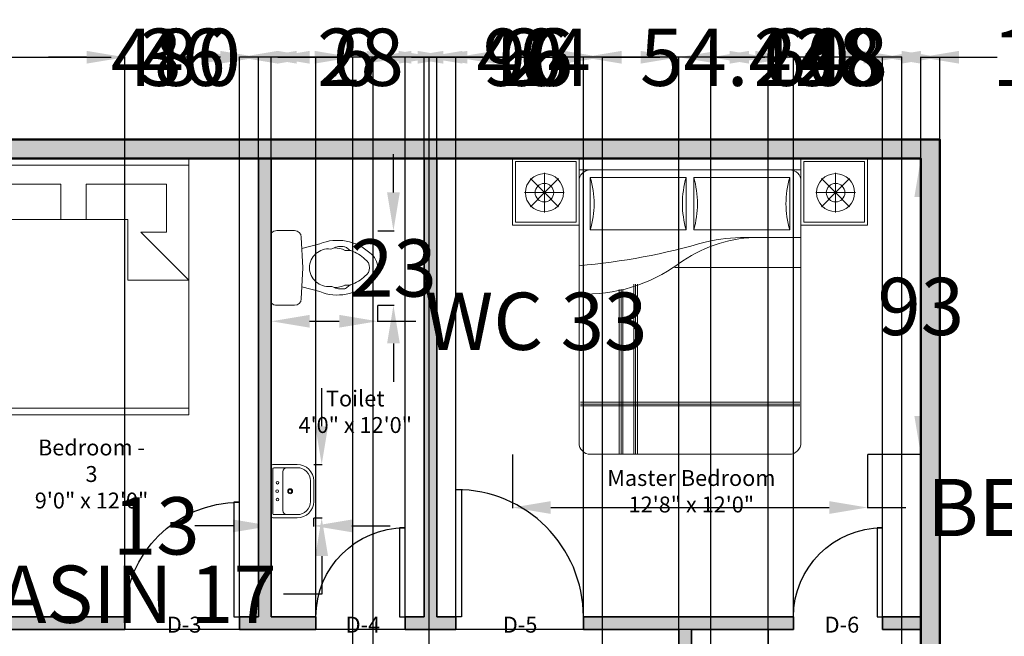
# Model space of a CAD drawing. Units: inches. Extents: x -478 to 256, y -93 to 343.
# Tile 4 of 5: x -211 to 98, y 149 to 343. Entities that reach past the tile are written whole.
import ezdxf

# ---------------------------------------------------------------- set-up
doc = ezdxf.new("R2010")
doc.units = ezdxf.units.IN
for name, color, linetype, lineweight in [('A-ANNO-DIMS', 2, 'Continuous', 18), ('A-ANNO-TEXT', 7, 'Continuous', 18), ('A-AREA-IDEN', 7, 'Continuous', 18), ('A-DOOR', 3, 'Continuous', 25), ('A-FLOR-CASE', 6, 'Continuous', 25), ('A-FLOR-FIXT', 9, 'Continuous', 18), ('A-WALL-PATT', 8, 'Continuous', 13), ('Furniture', 2, 'Continuous', 18), ('Inner Wall', 5, 'Continuous', 35), ('Outer Wall', 1, 'Continuous', 50)]:
    doc.layers.add(name, color=color, linetype=linetype, lineweight=lineweight)
doc.styles.get("Standard").update_dxf_attribs({"font": 'arial.ttf'})
doc.dimstyles.get("Standard").update_dxf_attribs({"dimtxt": 18, "dimasz": 12, "dimexe": 0.18, "dimexo": 0.0625, "dimgap": 0.09, "dimtad": 0, "dimtih": 1, "dimtoh": 1, "dimdec": 0, "dimzin": 0, "dimdsep": 46, "dimlunit": 3, "dimtxsty": 'Standard', "dimcen": 0.09, "dimadec": 0, "dimazin": 0, "dimtfac": 1, "dimtdec": 0, "dimtofl": 0, "dimtmove": 0, "dimatfit": 3, "dimfxl": 1, "dimtolj": 1, "dimtzin": 0, "dimarcsym": 0})

# ---------------------------------------------------------------- blocks, each defined once
blk = doc.blocks.new('*U2')
for p, q in [((0, 0), (0, -4)), ((36, 0), (36, -4))]:
    blk.add_line(p, q)
blk.add_lwpolyline([(0, 0), (0, 36), (1.75, 36), (1.75, 0)], close=True)
blk.add_arc((0, 0), 36, 0, 90)
blk = doc.blocks.new('*U3')
for p, q in [((0, 0), (0, -4)), ((40, 0), (40, -4))]:
    blk.add_line(p, q)
blk.add_lwpolyline([(0, 0), (0, 40), (1.75, 40), (1.75, 0)], close=True)
blk.add_arc((0, 0), 40, 0, 90)
blk = doc.blocks.new('*U4')
for p, q in [((0, 0), (0, -4)), ((28, 0), (28, -4))]:
    blk.add_line(p, q)
blk.add_lwpolyline([(0, 0), (0, 28), (1.75, 28), (1.75, 0)], close=True)
blk.add_arc((0, 0), 28, 0, 90)
blk = doc.blocks.new('A$C1308471B')
at = {"ltscale": 20}
for p, q in [((0, 0.4607), (0, 0.0186)), ((0.0354, 0.4793), (0.1495, 0.4793)), ((0.2013, 0.2397), (0.1923, 0.4384)), ((0.1957, 0.3639), (0.3109, 0.3953)), ((0.5021, 0.3528), (0.4724, 0.3528)), ((0.4982, 0.3575), (0.4822, 0.3709)), ((0.2013, 0.2397), (0.1923, 0.0409)), ((0.5021, 0.1304), (0.4724, 0.1304)), ((0.1959, 0.1193), (0.3109, 0.0879)), ((0.4982, 0.1257), (0.4822, 0.1123)), ((0.0354, 0), (0.1495, 0))]:
    blk.add_line(p, q, dxfattribs=at)
for centre, radius, start, end in [((0.006, 0.4607), 0.006, 136.52689, 180), ((0.0354, 0.4328), 0.0465, 90, 136.52689), ((0.1495, 0.4365), 0.0429, 2.57554, 90), ((0.4248, 0.1104), 0.3068, 47.41345, 111.79241), ((0.3654, 0.2416), 0.1206, 83.35226, 180), ((0.3823, 0.3868), 0.0255, 263.35226, 298.57415), ((0.4494, 0.2636), 0.1148, 79.39683, 118.57415), ((0.405, 0.2159), 0.153, 63.50202, 90.45216), ((0.4658, 0.3513), 0.0255, 50, 79.39683), ((0.5146, 0.377), 0.0255, 230, 251.38812), ((0.5021, 0.3273), 0.0255, 70.3751, 90), ((0.4248, 0.1104), 0.2558, 46.61198, 70.3751), ((0.5654, 0.2416), 0.116, 0, 54.71147), ((0.5654, 0.2416), 0.065, 0, 57.29738), ((0.3654, 0.2416), 0.1206, 180, 276.64774), ((0.5654, 0.2416), 0.065, 302.70262, 0), ((0.5654, 0.2416), 0.116, 305.28853, 0), ((0.4248, 0.3728), 0.3068, 248.20759, 312.58655), ((0.405, 0.2673), 0.153, 269.54784, 296.49798), ((0.5146, 0.1062), 0.0255, 108.61188, 130), ((0.5021, 0.1559), 0.0255, 270, 289.6249), ((0.4248, 0.3728), 0.2558, 289.6249, 313.38802), ((0.3823, 0.0964), 0.0255, 61.42585, 96.64774), ((0.4494, 0.2196), 0.1148, 241.42585, 280.60317), ((0.4658, 0.1319), 0.0255, 280.60317, 310), ((0.006, 0.0186), 0.006, 180, 223.47311), ((0.0354, 0.0465), 0.0465, 223.47311, 270), ((0.1495, 0.0429), 0.0429, 270, 357.42446)]:
    blk.add_arc(centre, radius, start, end, dxfattribs=at)
blk = doc.blocks.new('A$C57EA129C')
for p, q in [((0, 0.443), (0, 0.178)), ((0.016, 0.459), (0.563, 0.459)), ((0.036, 0.432), (0.036, 0.29)), ((0.045, 0.441), (0.535, 0.441)), ((0.544, 0.432), (0.544, 0.29)), ((0.579, 0.443), (0.579, 0.178)), ((0.08, 0.334), (0.499, 0.334)), ((0.036, 0.29), (0.036, 0.178)), ((0.544, 0.29), (0.544, 0.178)), ((0.178, 0.036), (0.401, 0.036)), ((0.178, 0), (0.401, 0))]:
    blk.add_line(p, q)
for centre, radius in [((0.198, 0.392), 0.0143), ((0.29, 0.396), 0.0156), ((0.381, 0.392), 0.0143), ((0.29, 0.255), 0.0267), ((0.29, 0.255), 0.0178)]:
    blk.add_circle(centre, radius)
for centre, radius, start, end in [((0.016, 0.443), 0.016, 90, 180), ((0.045, 0.432), 0.00891, 90, 180), ((0.535, 0.432), 0.00891, 0, 90), ((0.563, 0.443), 0.016, 0, 90), ((0.08, 0.29), 0.0445, 90, 180), ((0.499, 0.29), 0.0445, 0, 90), ((0.178, 0.178), 0.178, 180, 270), ((0.178, 0.178), 0.143, 180, 270), ((0.401, 0.178), 0.178, 270, 0), ((0.401, 0.178), 0.143, 270, 0)]:
    blk.add_arc(centre, radius, start, end)
blk = doc.blocks.new('KING-00')
for p, q in [((-0.8967, -0.947), (-0.8967, 0.8818)), ((0.6019, 0.8818), (0.6019, -0.4644)), ((1.0337, -0.947), (1.0337, 0.8818)), ((0.6019, 0.704), (0.8813, 0.704)), ((0.8813, 0.069), (0.8813, 0.704)), ((0.6019, 0.069), (0.8813, 0.069)), ((0.8813, -0.1342), (0.6019, -0.1342)), ((0.8813, -0.7692), (0.8813, -0.1342)), ((0.1193, -0.4644), (0.1193, -0.947)), ((0.6019, -0.4644), (0.1193, -0.4644)), ((0.1193, -0.947), (0.5003, -0.566)), ((0.5003, -0.7692), (0.5003, -0.566)), ((0.5003, -0.7692), (0.8813, -0.7692))]:
    blk.add_line(p, q)
blk.add_lwpolyline([(-0.9475, -0.947), (-0.9475, 0.8818), (1.0845, 0.8818), (1.0845, -0.947)], close=True)
blk = doc.blocks.new('A$C068671E6')
for p, q in [((0, 1.5502), (0, 2.0002)), ((0, 2.0002), (0.45, 2.0002)), ((0.45, 2.0002), (0.45, 1.5502)), ((1.9506, 2.0002), (1.9506, 1.5502)), ((2.4006, 2.0002), (1.9506, 2.0002)), ((2.4006, 1.5502), (2.4006, 2.0002)), ((0.02, 1.5702), (0.02, 1.9802)), ((0.02, 1.9802), (0.43, 1.9802)), ((0.43, 1.9802), (0.43, 1.5702)), ((1.9706, 1.9802), (1.9706, 1.5702)), ((2.3806, 1.9802), (1.9706, 1.9802)), ((2.3806, 1.5702), (2.3806, 1.9802)), ((0.216, 1.7702), (0.121, 1.8652)), ((0.216, 1.7702), (0.216, 1.9046)), ((0.216, 1.7702), (0.3111, 1.8652)), ((2.1846, 1.7702), (2.0895, 1.8652)), ((2.1846, 1.7702), (2.1846, 1.9046)), ((2.1846, 1.7702), (2.2796, 1.8652)), ((0.216, 1.7702), (0.0817, 1.7702)), ((0.216, 1.7702), (0.121, 1.6752)), ((0.216, 1.7702), (0.216, 1.6358)), ((0.216, 1.7702), (0.3111, 1.6752)), ((0.216, 1.7702), (0.3504, 1.7702)), ((2.1846, 1.7702), (2.0502, 1.7702)), ((2.1846, 1.7702), (2.0895, 1.6752)), ((2.1846, 1.7702), (2.1846, 1.6358)), ((2.1846, 1.7702), (2.3189, 1.7702)), ((2.1846, 1.7702), (2.2796, 1.6752)), ((0.45, 1.5502), (0, 1.5502)), ((0.43, 1.5702), (0.02, 1.5702)), ((1.9506, 1.5502), (2.4006, 1.5502)), ((1.9706, 1.5702), (2.3806, 1.5702)), ((0.8202, 1.1507), (0.8202, 0)), ((0.8322, 1.1507), (0.8322, 0)), ((0.8442, 1.1507), (0.8442, 0)), ((0.722, 1.1146), (0.722, 0)), ((0.734, 1.1146), (0.734, 0)), ((0.746, 1.1146), (0.746, 0)), ((0.4599, 0.3521), (1.9437, 0.3521)), ((0.4599, 0.3401), (1.9437, 0.3401)), ((0.4599, 0.3281), (1.9437, 0.3281))]:
    blk.add_line(p, q)
at = {"linetype": 'ByBlock'}
for p, q in [((0.45, 1.924), (0.45, 2.0002)), ((0.45, 2.0002), (1.9506, 2.0002)), ((1.9506, 1.924), (1.9506, 2.0002)), ((0.45, 1.924), (1.9506, 1.924)), ((1.1744, 1.8732), (0.5262, 1.8732)), ((0.5262, 1.8732), (0.5262, 1.5176)), ((1.1744, 1.5176), (1.1744, 1.8732)), ((1.8744, 1.8732), (1.2252, 1.8732)), ((1.2252, 1.8732), (1.2252, 1.5176)), ((1.8744, 1.5176), (1.8744, 1.8732)), ((0.45, 0.0762), (0.45, 1.8478)), ((1.9506, 1.8478), (1.9506, 0.08)), ((0.5262, 1.5176), (1.1744, 1.5176)), ((1.2252, 1.5176), (1.8744, 1.5176)), ((1.5747, 1.4668), (1.9506, 1.4668)), ((1.0982, 1.2636), (1.9506, 1.2636)), ((1.8706, 0), (0.5262, 0))]:
    blk.add_line(p, q, dxfattribs=at)
for centre, radius in [((0.216, 1.7702), 0.1285), ((2.1846, 1.7702), 0.1285), ((0.216, 1.7702), 0.0628), ((2.1846, 1.7702), 0.0628)]:
    blk.add_circle(centre, radius)
for centre, radius, start, end in [((0.5262, 1.8478), 0.0762, 90, 180), ((-0.0834, 1.6954), 0.635, 343.73979, 16.26021), ((1.784, 1.6954), 0.635, 163.73979, 196.26021), ((0.6156, 1.6954), 0.635, 343.73979, 16.26021), ((2.484, 1.6954), 0.635, 163.73979, 196.26021), ((1.8744, 1.8478), 0.0762, 0, 90), ((1.673, 0.534), 0.9338, 92.53978, 126.04031), ((1.5743, 0.2475), 1.2193, 89.98136, 102.46674), ((0.0692, 5.6598), 4.4006, 274.96238, 286.39109), ((0.4931, 2.1535), 1.07, 267.6917, 306.10591), ((0.5262, 0.0762), 0.0762, 180, 270), ((1.8706, 0.08), 0.08, 270, 0)]:
    blk.add_arc(centre, radius, start, end, dxfattribs=at)
blk = doc.blocks.new('*D23')
at = {"layer": 'A-ANNO-DIMS', "color": 0, "lineweight": -2, "transparency": 16777216}
for p, q in [((-131.86, 252.69), (-131.86, 247.56)), ((-98.5, 252.69), (-98.5, 247.56)), ((-119.86, 247.74), (-110.5, 247.74)), ((-98.5, 247.74), (-86.5, 247.74))]:
    blk.add_line(p, q, dxfattribs=at)
at = {"layer": 'A-ANNO-DIMS', "color": 0, "transparency": 16777216}
for points in [[(-119.86, 249.74), (-119.86, 245.74), (-131.86, 247.74)], [(-110.5, 249.74), (-110.5, 245.74), (-98.5, 247.74)]]:
    blk.add_solid(points, dxfattribs=at)
at = {"layer": 'Defpoints', "color": 0, "transparency": 16777216}
for p in [(-131.86, 252.75), (-98.5, 252.75), (-98.5, 247.74)]:
    blk.add_point(p, dxfattribs=at)
at = {"layer": 'A-ANNO-DIMS', "color": 0, "transparency": 16777216, "insert": (-48.71, 247.74), "char_height": 18, "attachment_point": 5}
blk.add_mtext('\\A1;WC 33', dxfattribs=at)
blk = doc.blocks.new('*D24')
at = {"layer": 'A-ANNO-DIMS', "color": 0, "lineweight": -2, "transparency": 16777216}
for p, q in [((-93.5, 288.21), (-93.5, 300.21)), ((-98.44, 276.21), (-93.32, 276.21)), ((-98.44, 252.75), (-93.32, 252.75)), ((-93.5, 240.75), (-93.5, 228.75))]:
    blk.add_line(p, q, dxfattribs=at)
at = {"layer": 'A-ANNO-DIMS', "color": 0, "transparency": 16777216}
for points in [[(-95.5, 288.21), (-91.5, 288.21), (-93.5, 276.21)], [(-95.5, 240.75), (-91.5, 240.75), (-93.5, 252.75)]]:
    blk.add_solid(points, dxfattribs=at)
at = {"layer": 'Defpoints', "color": 0, "transparency": 16777216}
for p in [(-98.5, 276.21), (-93.5, 276.21), (-98.5, 252.75)]:
    blk.add_point(p, dxfattribs=at)
at = {"layer": 'A-ANNO-DIMS', "color": 0, "transparency": 16777216, "insert": (-93.5, 264.48), "char_height": 18, "attachment_point": 5}
blk.add_mtext('\\A1;23', dxfattribs=at)
blk = doc.blocks.new('*D25')
at = {"layer": 'A-ANNO-DIMS', "color": 0, "lineweight": -2, "transparency": 16777216}
for p, q in [((-116.04, 214.73), (-116.04, 226.73)), ((-118.49, 202.73), (-115.86, 202.73)), ((-118.49, 185.95), (-115.86, 185.95)), ((-116.04, 173.95), (-116.04, 161.95)), ((-116.04, 161.95), (-128.04, 161.95))]:
    blk.add_line(p, q, dxfattribs=at)
at = {"layer": 'A-ANNO-DIMS', "color": 0, "transparency": 16777216}
for points in [[(-118.04, 214.73), (-114.04, 214.73), (-116.04, 202.73)], [(-118.04, 173.95), (-114.04, 173.95), (-116.04, 185.95)]]:
    blk.add_solid(points, dxfattribs=at)
at = {"layer": 'Defpoints', "color": 0, "transparency": 16777216}
for p in [(-118.56, 202.73), (-118.56, 185.95), (-116.04, 185.95)]:
    blk.add_point(p, dxfattribs=at)
at = {"layer": 'A-ANNO-DIMS', "color": 0, "transparency": 16777216, "insert": (-181.85, 161.95), "char_height": 18, "attachment_point": 5}
blk.add_mtext('\\A1;BASIN 17', dxfattribs=at)
blk = doc.blocks.new('*D26')
at = {"layer": 'A-ANNO-DIMS', "color": 0, "lineweight": -2, "transparency": 16777216}
for p, q in [((-131.86, 185.88), (-131.86, 183.25)), ((-118.56, 185.88), (-118.56, 183.25)), ((-143.86, 183.43), (-155.86, 183.43)), ((-106.56, 183.43), (-94.56, 183.43))]:
    blk.add_line(p, q, dxfattribs=at)
at = {"layer": 'A-ANNO-DIMS', "color": 0, "transparency": 16777216}
for points in [[(-143.86, 185.43), (-143.86, 181.43), (-131.86, 183.43)], [(-106.56, 185.43), (-106.56, 181.43), (-118.56, 183.43)]]:
    blk.add_solid(points, dxfattribs=at)
at = {"layer": 'Defpoints', "color": 0, "transparency": 16777216}
for p in [(-131.86, 185.95), (-118.56, 185.95), (-131.86, 183.43)]:
    blk.add_point(p, dxfattribs=at)
at = {"layer": 'A-ANNO-DIMS', "color": 0, "transparency": 16777216, "insert": (-167.99, 183.43), "char_height": 18, "attachment_point": 5}
blk.add_mtext('\\A1;13', dxfattribs=at)
blk = doc.blocks.new('*D27')
at = {"layer": 'A-ANNO-DIMS', "color": 0, "lineweight": -2, "transparency": 16777216}
for p, q in [((-56.12, 205.87), (-56.12, 189.02)), ((55.39, 205.87), (55.39, 189.02)), ((-44.12, 189.2), (43.39, 189.2)), ((55.39, 189.2), (67.39, 189.2))]:
    blk.add_line(p, q, dxfattribs=at)
at = {"layer": 'A-ANNO-DIMS', "color": 0, "transparency": 16777216}
for points in [[(-44.12, 191.2), (-44.12, 187.2), (-56.12, 189.2)], [(43.39, 191.2), (43.39, 187.2), (55.39, 189.2)]]:
    blk.add_solid(points, dxfattribs=at)
at = {"layer": 'Defpoints', "color": 0, "transparency": 16777216}
for p in [(-56.12, 205.93), (55.39, 205.93), (55.39, 189.2)]:
    blk.add_point(p, dxfattribs=at)
at = {"layer": 'A-ANNO-DIMS', "color": 0, "transparency": 16777216, "insert": (165.82, 189.2), "char_height": 18, "attachment_point": 5}
blk.add_mtext('\\A1;BED GROUP 112', dxfattribs=at)
blk = doc.blocks.new('*D28')
at = {"layer": 'A-ANNO-DIMS', "color": 0, "lineweight": -2, "transparency": 16777216}
for p, q in [((55.46, 298.84), (72.3, 298.84)), ((72.12, 286.84), (72.12, 261.67)), ((72.12, 217.93), (72.12, 243.1)), ((55.46, 205.93), (72.3, 205.93))]:
    blk.add_line(p, q, dxfattribs=at)
at = {"layer": 'A-ANNO-DIMS', "color": 0, "transparency": 16777216}
for points in [[(70.12, 286.84), (74.12, 286.84), (72.12, 298.84)], [(70.12, 217.93), (74.12, 217.93), (72.12, 205.93)]]:
    blk.add_solid(points, dxfattribs=at)
at = {"layer": 'Defpoints', "color": 0, "transparency": 16777216}
for p in [(55.39, 298.84), (72.12, 298.84), (55.39, 205.93)]:
    blk.add_point(p, dxfattribs=at)
at = {"layer": 'A-ANNO-DIMS', "color": 0, "transparency": 16777216, "insert": (72.12, 252.39), "char_height": 18, "attachment_point": 5}
blk.add_mtext('\\A1;93', dxfattribs=at)
blk = doc.blocks.new('*D31')
at = {"layer": 'A-ANNO-DIMS', "color": 0, "lineweight": -2, "transparency": 16777216}
for p, q in [((-401.86, 304.9), (-401.86, 330.89)), ((78.14, 304.9), (78.14, 330.89)), ((-389.86, 330.71), (-182.16, 330.71)), ((66.14, 330.71), (-141.55, 330.71))]:
    blk.add_line(p, q, dxfattribs=at)
at = {"layer": 'A-ANNO-DIMS', "color": 0, "transparency": 16777216}
for points in [[(-389.86, 332.71), (-389.86, 328.71), (-401.86, 330.71)], [(66.14, 332.71), (66.14, 328.71), (78.14, 330.71)]]:
    blk.add_solid(points, dxfattribs=at)
at = {"layer": 'Defpoints', "color": 0, "transparency": 16777216}
for p in [(78.14, 330.71), (-401.86, 304.84), (78.14, 304.84)]:
    blk.add_point(p, dxfattribs=at)
at = {"layer": 'A-ANNO-DIMS', "color": 0, "transparency": 16777216, "insert": (-161.86, 330.71), "char_height": 18, "attachment_point": 5}
blk.add_mtext('\\A1;480', dxfattribs=at)
blk = doc.blocks.new('*D44')
at = {"layer": 'A-ANNO-DIMS', "color": 0, "lineweight": -2, "transparency": 16777216}
for p, q in [((-177.855811, 154.903597), (-177.855811, 330.886097)), ((-141.855811, 154.903597), (-141.855811, 330.886097)), ((-189.855811, 330.706097), (-201.855811, 330.706097)), ((-129.855811, 330.706097), (-117.855811, 330.706097))]:
    blk.add_line(p, q, dxfattribs=at)
at = {"layer": 'A-ANNO-DIMS', "color": 0, "transparency": 16777216}
for points in [[(-189.855811, 332.706097), (-189.855811, 328.706097), (-177.855811, 330.706097)], [(-129.855811, 332.706097), (-129.855811, 328.706097), (-141.855811, 330.706097)]]:
    blk.add_solid(points, dxfattribs=at)
at = {"layer": 'Defpoints', "color": 0, "transparency": 16777216}
for p in [(-141.855811, 330.706097), (-177.855811, 154.841097), (-141.855811, 154.841097)]:
    blk.add_point(p, dxfattribs=at)
at = {"layer": 'A-ANNO-DIMS', "color": 0, "transparency": 16777216, "insert": (-159.855811, 330.706097), "char_height": 18, "attachment_point": 5}
blk.add_mtext('\\A1;36', dxfattribs=at)
blk = doc.blocks.new('*D45')
at = {"layer": 'A-ANNO-DIMS', "color": 0, "lineweight": -2, "transparency": 16777216}
for p, q in [((-141.86, 154.9), (-141.86, 330.89)), ((-135.86, 154.9), (-135.86, 330.89)), ((-153.86, 330.71), (-165.86, 330.71)), ((-123.86, 330.71), (-111.86, 330.71))]:
    blk.add_line(p, q, dxfattribs=at)
at = {"layer": 'A-ANNO-DIMS', "color": 0, "transparency": 16777216}
for points in [[(-153.86, 332.71), (-153.86, 328.71), (-141.86, 330.71)], [(-123.86, 332.71), (-123.86, 328.71), (-135.86, 330.71)]]:
    blk.add_solid(points, dxfattribs=at)
at = {"layer": 'Defpoints', "color": 0, "transparency": 16777216}
for p in [(-135.86, 330.71), (-141.86, 154.84), (-135.86, 154.84)]:
    blk.add_point(p, dxfattribs=at)
at = {"layer": 'A-ANNO-DIMS', "color": 0, "transparency": 16777216, "insert": (-105.82, 330.71), "char_height": 18, "attachment_point": 5}
blk.add_mtext('\\A1;6', dxfattribs=at)
blk = doc.blocks.new('*D46')
at = {"layer": 'A-ANNO-DIMS', "color": 0, "lineweight": -2, "transparency": 16777216}
for p, q in [((-117.855811, 154.903597), (-117.855811, 330.886097)), ((-89.855811, 154.903597), (-89.855811, 330.886097)), ((-129.855811, 330.706097), (-141.855811, 330.706097)), ((-77.855811, 330.706097), (-65.855811, 330.706097))]:
    blk.add_line(p, q, dxfattribs=at)
at = {"layer": 'A-ANNO-DIMS', "color": 0, "transparency": 16777216}
for points in [[(-129.855811, 332.706097), (-129.855811, 328.706097), (-117.855811, 330.706097)], [(-77.855811, 332.706097), (-77.855811, 328.706097), (-89.855811, 330.706097)]]:
    blk.add_solid(points, dxfattribs=at)
at = {"layer": 'Defpoints', "color": 0, "transparency": 16777216}
for p in [(-89.855811, 330.706097), (-117.855811, 154.841097), (-89.855811, 154.841097)]:
    blk.add_point(p, dxfattribs=at)
at = {"layer": 'A-ANNO-DIMS', "color": 0, "transparency": 16777216, "insert": (-103.855811, 330.706097), "char_height": 18, "attachment_point": 5}
blk.add_mtext('\\A1;28', dxfattribs=at)
blk = doc.blocks.new('*D47')
at = {"layer": 'A-ANNO-DIMS', "color": 0, "lineweight": -2, "transparency": 16777216}
for p, q in [((-89.86, 154.9), (-89.86, 330.89)), ((-83.86, 154.9), (-83.86, 330.89)), ((-101.86, 330.71), (-113.86, 330.71)), ((-71.86, 330.71), (-59.86, 330.71))]:
    blk.add_line(p, q, dxfattribs=at)
at = {"layer": 'A-ANNO-DIMS', "color": 0, "transparency": 16777216}
for points in [[(-101.86, 332.71), (-101.86, 328.71), (-89.86, 330.71)], [(-71.86, 332.71), (-71.86, 328.71), (-83.86, 330.71)]]:
    blk.add_solid(points, dxfattribs=at)
at = {"layer": 'Defpoints', "color": 0, "transparency": 16777216}
for p in [(-83.86, 330.71), (-89.86, 154.84), (-83.86, 154.84)]:
    blk.add_point(p, dxfattribs=at)
at = {"layer": 'A-ANNO-DIMS', "color": 0, "transparency": 16777216, "insert": (-53.82, 330.71), "char_height": 18, "attachment_point": 5}
blk.add_mtext('\\A1;6', dxfattribs=at)
blk = doc.blocks.new('*D48')
at = {"layer": 'A-ANNO-DIMS', "color": 0, "lineweight": -2, "transparency": 16777216}
for p, q in [((-73.855811, 154.903597), (-73.855811, 330.886097)), ((-33.855811, 154.903597), (-33.855811, 330.886097)), ((-85.855811, 330.706097), (-97.855811, 330.706097)), ((-21.855811, 330.706097), (-9.855811, 330.706097))]:
    blk.add_line(p, q, dxfattribs=at)
at = {"layer": 'A-ANNO-DIMS', "color": 0, "transparency": 16777216}
for points in [[(-85.855811, 332.706097), (-85.855811, 328.706097), (-73.855811, 330.706097)], [(-21.855811, 332.706097), (-21.855811, 328.706097), (-33.855811, 330.706097)]]:
    blk.add_solid(points, dxfattribs=at)
at = {"layer": 'Defpoints', "color": 0, "transparency": 16777216}
for p in [(-33.855811, 330.706097), (-73.855811, 154.841097), (-33.855811, 154.841097)]:
    blk.add_point(p, dxfattribs=at)
at = {"layer": 'A-ANNO-DIMS', "color": 0, "transparency": 16777216, "insert": (-53.855811, 330.706097), "char_height": 18, "attachment_point": 5}
blk.add_mtext('\\A1;40', dxfattribs=at)
blk = doc.blocks.new('*D49')
at = {"layer": 'A-ANNO-DIMS', "color": 0, "lineweight": -2, "transparency": 16777216}
for p, q in [((-79.86, 154.9), (-79.86, 330.89)), ((-73.86, 154.9), (-73.86, 330.89)), ((-91.86, 330.71), (-103.86, 330.71)), ((-61.86, 330.71), (-49.86, 330.71))]:
    blk.add_line(p, q, dxfattribs=at)
at = {"layer": 'A-ANNO-DIMS', "color": 0, "transparency": 16777216}
for points in [[(-91.86, 332.71), (-91.86, 328.71), (-79.86, 330.71)], [(-61.86, 332.71), (-61.86, 328.71), (-73.86, 330.71)]]:
    blk.add_solid(points, dxfattribs=at)
at = {"layer": 'Defpoints', "color": 0, "transparency": 16777216}
for p in [(-73.86, 330.71), (-79.86, 154.84), (-73.86, 154.84)]:
    blk.add_point(p, dxfattribs=at)
at = {"layer": 'A-ANNO-DIMS', "color": 0, "transparency": 16777216, "insert": (-43.82, 330.71), "char_height": 18, "attachment_point": 5}
blk.add_mtext('\\A1;6', dxfattribs=at)
blk = doc.blocks.new('*D50')
at = {"layer": 'A-ANNO-DIMS', "color": 0, "lineweight": -2, "transparency": 16777216}
for p, q in [((32.144189, 154.903597), (32.144189, 330.886097)), ((60.144189, 154.903597), (60.144189, 330.886097)), ((20.144189, 330.706097), (8.144189, 330.706097)), ((72.144189, 330.706097), (84.144189, 330.706097))]:
    blk.add_line(p, q, dxfattribs=at)
at = {"layer": 'A-ANNO-DIMS', "color": 0, "transparency": 16777216}
for points in [[(20.144189, 332.706097), (20.144189, 328.706097), (32.144189, 330.706097)], [(72.144189, 332.706097), (72.144189, 328.706097), (60.144189, 330.706097)]]:
    blk.add_solid(points, dxfattribs=at)
at = {"layer": 'Defpoints', "color": 0, "transparency": 16777216}
for p in [(60.144189, 330.706097), (32.144189, 154.841097), (60.144189, 154.841097)]:
    blk.add_point(p, dxfattribs=at)
at = {"layer": 'A-ANNO-DIMS', "color": 0, "transparency": 16777216, "insert": (46.144189, 330.706097), "char_height": 18, "attachment_point": 5}
blk.add_mtext('\\A1;28', dxfattribs=at)
blk = doc.blocks.new('*D51')
at = {"layer": 'A-ANNO-DIMS', "color": 0, "lineweight": -2, "transparency": 16777216}
for p, q in [((60.14, 154.9), (60.14, 330.89)), ((72.14, 154.9), (72.14, 330.89)), ((48.14, 330.71), (36.14, 330.71)), ((84.14, 330.71), (96.14, 330.71))]:
    blk.add_line(p, q, dxfattribs=at)
at = {"layer": 'A-ANNO-DIMS', "color": 0, "transparency": 16777216}
for points in [[(48.14, 332.71), (48.14, 328.71), (60.14, 330.71)], [(84.14, 332.71), (84.14, 328.71), (72.14, 330.71)]]:
    blk.add_solid(points, dxfattribs=at)
at = {"layer": 'Defpoints', "color": 0, "transparency": 16777216}
for p in [(72.14, 330.71), (60.14, 154.84), (72.14, 154.84)]:
    blk.add_point(p, dxfattribs=at)
at = {"layer": 'A-ANNO-DIMS', "color": 0, "transparency": 16777216, "insert": (108.19, 330.71), "char_height": 18, "attachment_point": 5}
blk.add_mtext('\\A1;12', dxfattribs=at)
blk = doc.blocks.new('*D53')
at = {"layer": 'A-ANNO-DIMS', "color": 0, "lineweight": -2, "transparency": 16777216}
for p, q in [((-106.28, 101.01), (-106.28, 330.89)), ((-82.28, 101.01), (-82.28, 330.89)), ((-118.28, 330.71), (-130.28, 330.71)), ((-70.28, 330.71), (-58.28, 330.71))]:
    blk.add_line(p, q, dxfattribs=at)
at = {"layer": 'A-ANNO-DIMS', "color": 0, "transparency": 16777216}
for points in [[(-118.28, 332.71), (-118.28, 328.71), (-106.28, 330.71)], [(-70.28, 332.71), (-70.28, 328.71), (-82.28, 330.71)]]:
    blk.add_solid(points, dxfattribs=at)
at = {"layer": 'Defpoints', "color": 0, "transparency": 16777216}
for p in [(-82.28, 330.71), (-106.28, 100.95), (-82.28, 100.95)]:
    blk.add_point(p, dxfattribs=at)
at = {"layer": 'A-ANNO-DIMS', "color": 0, "transparency": 16777216, "insert": (-45.18, 330.71), "char_height": 18, "attachment_point": 5}
blk.add_mtext('\\A1;24', dxfattribs=at)
blk = doc.blocks.new('*D56')
at = {"layer": 'A-ANNO-DIMS', "color": 0, "lineweight": -2, "transparency": 16777216}
for p, q in [((-135.86, 298.9), (-135.86, 330.89)), ((-131.86, 298.9), (-131.86, 330.89)), ((-147.86, 330.71), (-159.86, 330.71)), ((-119.86, 330.71), (-107.86, 330.71))]:
    blk.add_line(p, q, dxfattribs=at)
at = {"layer": 'A-ANNO-DIMS', "color": 0, "transparency": 16777216}
for points in [[(-147.86, 332.71), (-147.86, 328.71), (-135.86, 330.71)], [(-119.86, 332.71), (-119.86, 328.71), (-131.86, 330.71)]]:
    blk.add_solid(points, dxfattribs=at)
at = {"layer": 'Defpoints', "color": 0, "transparency": 16777216}
for p in [(-135.86, 330.71), (-135.86, 298.84), (-131.86, 298.84)]:
    blk.add_point(p, dxfattribs=at)
at = {"layer": 'A-ANNO-DIMS', "color": 0, "transparency": 16777216, "insert": (-166.17, 330.71), "char_height": 18, "attachment_point": 5}
blk.add_mtext('\\A1;4', dxfattribs=at)
blk = doc.blocks.new('*D57')
at = {"layer": 'A-ANNO-DIMS', "color": 0, "lineweight": -2, "transparency": 16777216}
for p, q in [((-99.86, -25.1), (-99.86, 330.89)), ((-3.86, -25.1), (-3.86, 330.89)), ((-87.86, 330.71), (-64.83, 330.71)), ((-15.86, 330.71), (-38.88, 330.71))]:
    blk.add_line(p, q, dxfattribs=at)
at = {"layer": 'A-ANNO-DIMS', "color": 0, "transparency": 16777216}
for points in [[(-87.86, 332.71), (-87.86, 328.71), (-99.86, 330.71)], [(-15.86, 332.71), (-15.86, 328.71), (-3.86, 330.71)]]:
    blk.add_solid(points, dxfattribs=at)
at = {"layer": 'Defpoints', "color": 0, "transparency": 16777216}
for p in [(-3.86, 330.71), (-99.86, -25.16), (-3.86, -25.16)]:
    blk.add_point(p, dxfattribs=at)
at = {"layer": 'A-ANNO-DIMS', "color": 0, "transparency": 16777216, "insert": (-51.86, 330.71), "char_height": 18, "attachment_point": 5}
blk.add_mtext('\\A1;96', dxfattribs=at)
blk = doc.blocks.new('*D60')
at = {"layer": 'A-ANNO-DIMS', "color": 0, "lineweight": -2, "transparency": 16777216}
for p, q in [((-27.86, 18.9), (-27.86, 330.89)), ((-3.86, 18.9), (-3.86, 330.89)), ((-39.86, 330.71), (-51.86, 330.71)), ((8.14, 330.71), (20.14, 330.71))]:
    blk.add_line(p, q, dxfattribs=at)
at = {"layer": 'A-ANNO-DIMS', "color": 0, "transparency": 16777216}
for points in [[(-39.86, 332.71), (-39.86, 328.71), (-27.86, 330.71)], [(8.14, 332.71), (8.14, 328.71), (-3.86, 330.71)]]:
    blk.add_solid(points, dxfattribs=at)
at = {"layer": 'Defpoints', "color": 0, "transparency": 16777216}
for p in [(-3.86, 330.71), (-27.86, 18.84), (-3.86, 18.84)]:
    blk.add_point(p, dxfattribs=at)
at = {"layer": 'A-ANNO-DIMS', "color": 0, "transparency": 16777216, "insert": (33.24, 330.71), "char_height": 18, "attachment_point": 5}
blk.add_mtext('\\A1;24', dxfattribs=at)
blk = doc.blocks.new('*D62')
at = {"layer": 'A-ANNO-DIMS', "color": 0, "lineweight": -2, "transparency": 16777216}
for p, q in [((-82.28, 53.01), (-82.28, 330.89)), ((-27.86, 18.9), (-27.86, 330.89)), ((-70.28, 330.71), (-39.86, 330.71)), ((-27.86, 330.71), (-15.86, 330.71))]:
    blk.add_line(p, q, dxfattribs=at)
at = {"layer": 'A-ANNO-DIMS', "color": 0, "transparency": 16777216}
for points in [[(-70.28, 332.71), (-70.28, 328.71), (-82.28, 330.71)], [(-39.86, 332.71), (-39.86, 328.71), (-27.86, 330.71)]]:
    blk.add_solid(points, dxfattribs=at)
at = {"layer": 'Defpoints', "color": 0, "transparency": 16777216}
for p in [(-27.86, 330.71), (-82.28, 52.95), (-27.86, 18.84)]:
    blk.add_point(p, dxfattribs=at)
at = {"layer": 'A-ANNO-DIMS', "color": 0, "transparency": 16777216, "insert": (14.6, 330.71), "char_height": 18, "attachment_point": 5}
blk.add_mtext('\\A1;54.43', dxfattribs=at)
blk = doc.blocks.new('*D65')
at = {"layer": 'A-ANNO-DIMS', "color": 0, "lineweight": -2, "transparency": 16777216}
for p, q in [((24.144189, 90.903597), (24.144189, 330.886097)), ((72.144189, 90.903597), (72.144189, 330.886097)), ((12.144189, 330.706097), (0.144189, 330.706097)), ((84.144189, 330.706097), (96.144189, 330.706097))]:
    blk.add_line(p, q, dxfattribs=at)
at = {"layer": 'A-ANNO-DIMS', "color": 0, "transparency": 16777216}
for points in [[(12.144189, 332.706097), (12.144189, 328.706097), (24.144189, 330.706097)], [(84.144189, 332.706097), (84.144189, 328.706097), (72.144189, 330.706097)]]:
    blk.add_solid(points, dxfattribs=at)
at = {"layer": 'Defpoints', "color": 0, "transparency": 16777216}
for p in [(72.144189, 330.706097), (24.144189, 90.841097), (72.144189, 90.841097)]:
    blk.add_point(p, dxfattribs=at)
at = {"layer": 'A-ANNO-DIMS', "color": 0, "transparency": 16777216, "insert": (48.144189, 330.706097), "char_height": 18, "attachment_point": 5}
blk.add_mtext('\\A1;48', dxfattribs=at)
blk = doc.blocks.new('*D66')
at = {"layer": 'A-ANNO-DIMS', "color": 0, "lineweight": -2, "transparency": 16777216}
for p, q in [((24.08, 150.84), (-427.9, 150.84)), ((-427.72, 138.84), (-427.72, 130.12)), ((-427.72, 102.84), (-427.72, 111.56)), ((24.08, 90.84), (-427.9, 90.84))]:
    blk.add_line(p, q, dxfattribs=at)
at = {"layer": 'A-ANNO-DIMS', "color": 0, "transparency": 16777216}
for points in [[(-429.72, 138.84), (-425.72, 138.84), (-427.72, 150.84)], [(-429.72, 102.84), (-425.72, 102.84), (-427.72, 90.84)]]:
    blk.add_solid(points, dxfattribs=at)
at = {"layer": 'Defpoints', "color": 0, "transparency": 16777216}
for p in [(-427.72, 150.84), (24.14, 150.84), (24.14, 90.84)]:
    blk.add_point(p, dxfattribs=at)
at = {"layer": 'A-ANNO-DIMS', "color": 0, "transparency": 16777216, "insert": (-427.72, 120.84), "char_height": 18, "attachment_point": 5}
blk.add_mtext('\\A1;60', dxfattribs=at)
blk = doc.blocks.new('*D67')
at = {"layer": 'A-ANNO-DIMS', "color": 0, "lineweight": -2, "transparency": 16777216}
for p, q in [((6.14, -25.1), (6.14, 330.89)), ((66.14, -25.1), (66.14, 330.89)), ((18.14, 330.71), (23.14, 330.71)), ((54.14, 330.71), (49.14, 330.71))]:
    blk.add_line(p, q, dxfattribs=at)
at = {"layer": 'A-ANNO-DIMS', "color": 0, "transparency": 16777216}
for points in [[(18.14, 332.71), (18.14, 328.71), (6.14, 330.71)], [(54.14, 332.71), (54.14, 328.71), (66.14, 330.71)]]:
    blk.add_solid(points, dxfattribs=at)
at = {"layer": 'Defpoints', "color": 0, "transparency": 16777216}
for p in [(66.14, 330.71), (6.14, -25.16), (66.14, -25.16)]:
    blk.add_point(p, dxfattribs=at)
at = {"layer": 'A-ANNO-DIMS', "color": 0, "transparency": 16777216, "insert": (36.14, 330.71), "char_height": 18, "attachment_point": 5}
blk.add_mtext('\\A1;60', dxfattribs=at)

msp = doc.modelspace()

# ---------------------------------------------------------------- hatches: boundary and pattern name
at = {"layer": 'A-WALL-PATT'}
h = msp.add_hatch(color=256, dxfattribs=at)
h.dxf.hatch_style = 1
h.paths.add_polyline_path([(-395.856, 298.841), (72.144, 298.841), (72.144, 20.841), (78.144, 20.841), (78.144, 304.841), (-401.856, 304.841), (-401.856, -55.159), (-215.856, -55.159), (-215.856, -49.159), (-395.856, -49.159)])
h.paths.add_polyline_path([(78.144, -15.159), (72.144, -15.159), (72.144, -49.159), (-179.856, -49.159), (-179.856, -55.159), (78.144, -55.159)], flags=17)
h = msp.add_hatch(color=256, dxfattribs=at)
h.dxf.hatch_style = 1
h.paths.add_polyline_path([(-329.856, 154.841), (-395.856, 154.841), (-395.856, 150.841), (-329.856, 150.841)])
h.paths.add_polyline_path([(-177.856, 154.841), (-243.856, 154.841), (-243.856, 160.841), (-247.856, 160.841), (-247.856, 154.841), (-283.856, 154.841), (-283.856, 224.841), (-247.856, 224.841), (-247.856, 218.841), (-243.856, 218.841), (-243.856, 298.841), (-247.856, 298.841), (-247.856, 228.841), (-283.856, 228.841), (-283.856, 234.841), (-287.856, 234.841), (-287.856, 154.841), (-293.856, 154.841), (-293.856, 150.841), (-177.856, 150.841)])
h.paths.add_polyline_path([(-283.856, 298.841), (-287.856, 298.841), (-287.856, 292.841), (-283.856, 292.841)], flags=17)
h.paths.add_polyline_path([(-131.856, 298.841), (-135.856, 298.841), (-135.856, 154.841), (-141.856, 154.841), (-141.856, 150.841), (-117.856, 150.841), (-117.856, 154.841), (-131.856, 154.841)])
h.paths.add_polyline_path([(-79.856, 298.841), (-83.856, 298.841), (-83.856, 154.841), (-89.856, 154.841), (-89.856, 150.841), (-73.856, 150.841), (-73.856, 154.841), (-79.856, 154.841)])
h.paths.add_polyline_path([(32.144, 154.841), (-33.856, 154.841), (-33.856, 150.841), (-3.856, 150.841), (-3.856, 12.841), (0.144, 12.841), (0.144, 62.841), (72.144, 62.841), (72.144, 66.841), (0.144, 66.841), (0.144, 150.841), (32.144, 150.841)])
h.paths.add_polyline_path([(72.144, 154.841), (60.144, 154.841), (60.144, 150.841), (72.144, 150.841)], flags=17)
h.paths.add_polyline_path([(6.144, -21.159), (0.144, -21.159), (0.144, -15.159), (-3.856, -15.159), (-3.856, -49.159), (0.144, -49.159), (0.144, -25.159), (6.144, -25.159)])
h.paths.add_polyline_path([(72.144, -21.159), (66.144, -21.159), (66.144, -25.159), (72.144, -25.159)])

# ---------------------------------------------------------------- linework, layer by layer
at = {"layer": 'A-FLOR-CASE'}
msp.add_line((24.144, 150.841), (24.144, 90.841), dxfattribs=at)
at = {"layer": 'Inner Wall'}
for p, q in [((-135.856, 298.841), (-135.856, 154.841)), ((-131.856, 298.841), (-131.856, 154.841)), ((-83.856, 298.841), (-83.856, 154.841)), ((-79.856, 298.841), (-79.856, 154.841)), ((-243.856, 154.841), (-177.856, 154.841)), ((-177.856, 150.841), (-177.856, 154.841)), ((-141.856, 150.841), (-141.856, 154.841)), ((-141.856, 154.841), (-135.856, 154.841)), ((-131.856, 154.841), (-117.856, 154.841)), ((-117.856, 154.841), (-117.856, 150.841)), ((-89.856, 154.841), (-89.856, 150.841)), ((-89.856, 154.841), (-83.856, 154.841)), ((-79.856, 154.841), (-73.856, 154.841)), ((-73.856, 154.841), (-73.856, 150.841)), ((-33.856, 154.841), (-33.856, 150.841)), ((-33.856, 154.841), (32.144, 154.841)), ((32.144, 154.841), (32.144, 150.841)), ((60.144, 154.841), (60.144, 150.841)), ((60.144, 154.841), (72.144, 154.841)), ((-293.856, 150.841), (-177.856, 150.841)), ((-141.856, 150.841), (-117.856, 150.841)), ((-89.856, 150.841), (-73.856, 150.841)), ((-33.856, 150.841), (-3.856, 150.841)), ((-3.856, 150.841), (-3.856, 12.841)), ((0.144, 150.841), (0.144, 66.841)), ((0.144, 150.841), (32.144, 150.841)), ((60.144, 150.841), (72.144, 150.841))]:
    msp.add_line(p, q, dxfattribs=at)
at = {"layer": 'Outer Wall'}
for p, q in [((-395.856, 298.841), (72.144, 298.841)), ((72.144, 298.841), (72.144, 20.841))]:
    msp.add_line(p, q, dxfattribs=at)
msp.add_lwpolyline([(-215.856, -55.159), (-401.856, -55.159), (-401.856, 304.841), (78.144, 304.841), (78.144, 20.841)], dxfattribs=at)

# ---------------------------------------------------------------- block references
at = {"layer": 'A-DOOR'}
msp.add_blockref('*U3', (-73.856, 154.841), dxfattribs=at)
at = {"layer": 'A-DOOR', "xscale": -1}
for name, p in [('*U2', (-141.856, 154.841)), ('*U4', (-89.856, 154.841)), ('*U4', (60.144, 154.841))]:
    msp.add_blockref(name, p, dxfattribs=at)
at = {"layer": 'A-FLOR-FIXT', "xscale": 48.95497407897215, "yscale": 48.95497407897215, "zscale": 48.95497407897215}
msp.add_blockref('A$C1308471B', (-131.856, 252.748), dxfattribs=at)
at = {"layer": 'A-FLOR-FIXT', "xscale": -28.98333223671166, "yscale": 28.98333223671166, "zscale": 28.98333223671166, "rotation": 90}
msp.add_blockref('A$C57EA129C', (-118.556, 202.731), dxfattribs=at)
at = {"layer": 'Furniture', "xscale": 39.60249106241186, "yscale": 39.60249106241186, "zscale": 39.60249106241186, "rotation": 89.99999999999999}
msp.add_blockref('KING-00', (-195.282, 255.892), dxfattribs=at)
at = {"layer": 'Furniture', "xscale": 46.45082573670141, "yscale": 46.45082573670141, "zscale": 46.45082573670141}
msp.add_blockref('A$C068671E6', (-56.116, 205.93), dxfattribs=at)

# ---------------------------------------------------------------- texts
at = {"layer": 'A-ANNO-TEXT', "char_height": 5, "attachment_point": 3}
for s, insert in [('\\pxqc;{\\fTimes New Roman|b0|i0|c0|p18;D-3}', (-149.726, 154.888)), ('\\pxqc;{\\fTimes New Roman|b0|i0|c0|p18;D-4}', (-93.588, 154.888)), ('\\pxqc;{\\fTimes New Roman|b0|i0|c0|p18;D-5}', (-44.209, 154.888)), ('\\pxqc;{\\fTimes New Roman|b0|i0|c0|p18;D-6}', (56.852, 154.888))]:
    msp.add_mtext_dynamic_manual_height_columns(s, width=19.01487, gutter_width=12.5, heights=[0], dxfattribs=dict(at, insert=insert))
at = {"layer": 'A-AREA-IDEN', "char_height": 5, "attachment_point": 3}
for s, width, insert in [('\\pxqc;{\\fTimes New Roman|b0|i0|c0|p18;Toilet\\P4\'0" x 12\'0"}', 37.20338, (-86.903, 225.968)), ('\\pxqc;{\\fTimes New Roman|b0|i0|c0|p18;Bedroom - 3\\P9\'0" x 12\'0"}', 37.20338, (-169.725, 210.568)), ('\\pxqc;{\\fTimes New Roman|b0|i0|c0|p18;Master Bedroom\\P12\'8" x 12\'0"}', 65.74278, (32.931, 200.986))]:
    msp.add_mtext_dynamic_manual_height_columns(s, width=width, gutter_width=12.5, heights=[0], dxfattribs=dict(at, insert=insert))

# ---------------------------------------------------------------- dimensions: what is measured, and where the dimension line sits
at = {"layer": 'A-ANNO-DIMS'}
for base, p1, p2, override, picture, middle in [((78.144, 330.706), (-401.856, 304.841), (78.144, 304.841), {"dimdec": 0, "dimlfac": 1, "dimrnd": 0, "dimzin": 0, "dimdsep": 46, "dimlunit": 2}, '*D31', (-161.856, 330.706)), ((-141.856, 330.706), (-177.856, 154.841), (-141.856, 154.841), {"dimdec": 0, "dimlfac": 1, "dimrnd": 0, "dimzin": 0, "dimdsep": 46, "dimlunit": 2}, '*D44', (-159.856, 330.706)), ((-135.856, 330.706), (-131.856, 298.841), (-135.856, 298.841), {"dimdec": 0, "dimlfac": 1, "dimrnd": 0, "dimzin": 0, "dimdsep": 46, "dimlunit": 2}, '*D56', (-166.171, 330.706)), ((-135.856, 330.706), (-141.856, 154.841), (-135.856, 154.841), {"dimdec": 0, "dimlfac": 1, "dimrnd": 0, "dimzin": 0, "dimdsep": 46, "dimlunit": 2}, '*D45', (-105.823, 330.706)), ((-89.856, 330.706), (-117.856, 154.841), (-89.856, 154.841), {"dimdec": 0, "dimlfac": 1, "dimrnd": 0, "dimzin": 0, "dimdsep": 46, "dimlunit": 2}, '*D46', (-103.856, 330.706)), ((-82.284, 330.706), (-106.284, 100.949), (-82.284, 100.949), {"dimdec": 0, "dimlfac": 1, "dimrnd": 0, "dimzin": 0, "dimdsep": 46, "dimlunit": 2}, '*D53', (-45.185, 330.706)), ((-83.856, 330.706), (-89.856, 154.841), (-83.856, 154.841), {"dimdec": 0, "dimlfac": 1, "dimrnd": 0, "dimzin": 0, "dimdsep": 46, "dimlunit": 2}, '*D47', (-53.823, 330.706)), ((-73.856, 330.706), (-79.856, 154.841), (-73.856, 154.841), {"dimdec": 0, "dimlfac": 1, "dimrnd": 0, "dimzin": 0, "dimdsep": 46, "dimlunit": 2}, '*D49', (-43.823, 330.706)), ((-3.856, 330.706), (-99.856, -25.159), (-3.856, -25.159), {"dimdec": 0, "dimlfac": 1, "dimrnd": 0, "dimzin": 0, "dimdsep": 46, "dimlunit": 2}, '*D57', (-51.856, 330.706)), ((-33.856, 330.706), (-73.856, 154.841), (-33.856, 154.841), {"dimdec": 0, "dimlfac": 1, "dimrnd": 0, "dimzin": 0, "dimdsep": 46, "dimlunit": 2}, '*D48', (-53.856, 330.706)), ((-27.856, 330.706), (-82.284, 52.949), (-27.856, 18.841), {"dimdec": 2, "dimlfac": 1, "dimrnd": 0, "dimzin": 0, "dimdsep": 46, "dimlunit": 2}, '*D62', (14.605, 330.706)), ((-3.856, 330.706), (-27.856, 18.841), (-3.856, 18.841), {"dimdec": 0, "dimlfac": 1, "dimrnd": 0, "dimzin": 0, "dimdsep": 46, "dimlunit": 2}, '*D60', (33.243, 330.706)), ((72.144, 330.706), (24.144, 90.841), (72.144, 90.841), {"dimdec": 0, "dimlfac": 1, "dimrnd": 0, "dimzin": 0, "dimdsep": 46, "dimlunit": 2}, '*D65', (48.144, 330.706)), ((66.144, 330.706), (6.144, -25.159), (66.144, -25.159), {"dimdec": 0, "dimlfac": 1, "dimrnd": 0, "dimzin": 0, "dimdsep": 46, "dimlunit": 2}, '*D67', (36.144, 330.706)), ((60.144, 330.706), (32.144, 154.841), (60.144, 154.841), {"dimdec": 0, "dimlfac": 1, "dimrnd": 0, "dimzin": 0, "dimdsep": 46, "dimlunit": 2}, '*D50', (46.144, 330.706)), ((72.144, 330.706), (60.144, 154.841), (72.144, 154.841), {"dimdec": 0, "dimlfac": 1, "dimrnd": 0, "dimzin": 0, "dimdsep": 46, "dimlunit": 2}, '*D51', (108.187, 330.706))]:
    dim = msp.add_linear_dim(base=base, p1=p1, p2=p2, dimstyle='Standard', override=override, dxfattribs=at)
    dim.commit()
    dim.dimension.update_dxf_attribs({"geometry": picture, "text_midpoint": middle})
for base, p1, p2, angle, picture, middle in [((-93.496, 276.215), (-98.499, 252.748), (-98.499, 276.215), 90, '*D24', (-93.496, 264.481)), ((72.12, 298.841), (55.394, 205.93), (55.394, 298.841), 90, '*D28', (72.12, 252.386)), ((-131.856, 183.427), (-118.556, 185.945), (-131.856, 185.945), 180, '*D26', (-167.991, 183.427)), ((-427.721, 150.841), (24.144, 90.841), (24.144, 150.841), 90, '*D66', (-427.721, 120.841))]:
    dim = msp.add_linear_dim(base=base, p1=p1, p2=p2, angle=angle, dimstyle='Standard', override={"dimdec": 0, "dimlfac": 1, "dimrnd": 0, "dimzin": 0, "dimdsep": 46, "dimlunit": 2}, dxfattribs=at)
    dim.commit()
    dim.dimension.update_dxf_attribs({"geometry": picture, "text_midpoint": middle})
for base, p1, p2, text, picture, middle in [((-98.499, 247.745), (-131.856, 252.748), (-98.499, 252.748), 'WC <>', '*D23', (-48.709, 247.745)), ((55.394, 189.204), (-56.116, 205.93), (55.394, 205.93), 'BED GROUP <>', '*D27', (165.821, 189.204))]:
    dim = msp.add_linear_dim(base=base, p1=p1, p2=p2, text=text, dimstyle='Standard', override={"dimdec": 0, "dimlfac": 1, "dimrnd": 0, "dimzin": 0, "dimdsep": 46, "dimlunit": 2}, dxfattribs=at)
    dim.commit()
    dim.dimension.update_dxf_attribs({"geometry": picture, "text_midpoint": middle})
dim = msp.add_linear_dim(base=(-116.039, 185.945), p1=(-118.556, 202.731), p2=(-118.556, 185.945), angle=270, text='BASIN <>', dimstyle='Standard', override={"dimdec": 0, "dimlfac": 1, "dimrnd": 0, "dimzin": 0, "dimdsep": 46, "dimlunit": 2}, dxfattribs=at)
dim.commit()
dim.dimension.update_dxf_attribs({"geometry": '*D25', "text_midpoint": (-181.846, 161.945)})

doc.saveas('drawing.dxf')
